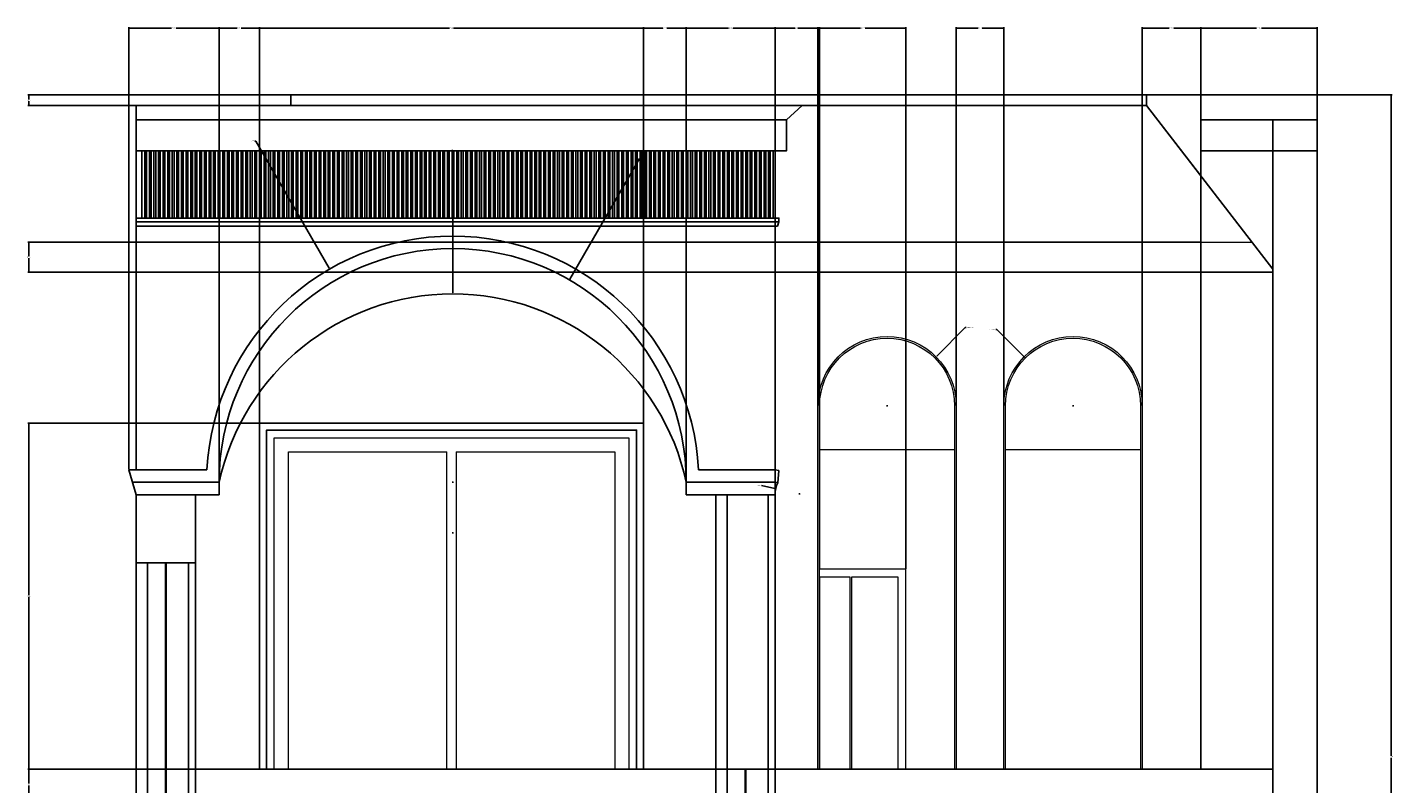
# Model space of a CAD drawing. Units: feet. Extents: x 2352 to 2983, y 950 to 1233.
# Tile 5 of 5: x 2718 to 2983, y 1086 to 1233. Entities that reach past the tile are written whole.
import ezdxf

# ---------------------------------------------------------------- set-up
doc = ezdxf.new("R2010")
doc.units = ezdxf.units.FT
for name, color, linetype, lineweight in [('A-ANNO-DIMS', 2, 'Continuous', 18), ('A-ELEV', 7, 'Continuous', 25), ('A-GLAZ', 4, 'Continuous', 18)]:
    doc.layers.add(name, color=color, linetype=linetype, lineweight=lineweight)
doc.styles.get("Standard").update_dxf_attribs({"font": 'arial.ttf'})
doc.dimstyles.get("Standard").update_dxf_attribs({"dimtxt": 0.18, "dimasz": 0.18, "dimexe": 0.18, "dimexo": 0.0625, "dimgap": 0.09, "dimtad": 0, "dimtih": 1, "dimtoh": 1, "dimdec": 1, "dimzin": 0, "dimdsep": 46, "dimlunit": 3, "dimtxsty": 'Standard', "dimcen": 0.09, "dimadec": 0, "dimazin": 0, "dimtfac": 1, "dimtdec": 1, "dimtofl": 0, "dimtmove": 0, "dimatfit": 3, "dimfxl": 1, "dimtolj": 1, "dimtzin": 0, "dimarcsym": 0})

# ---------------------------------------------------------------- blocks, each defined once
blk = doc.blocks.new('*D30')
at = {"layer": 'A-ANNO-DIMS', "color": 0, "lineweight": -2, "transparency": 16777216}
for p, q in [((2934.99, 1219.82), (2982.56, 1219.82)), ((2982.38, 1219.64), (2982.38, 1091.6)), ((2982.38, 963.19), (2982.38, 1091.23)), ((2969.32, 963.01), (2982.56, 963.01))]:
    blk.add_line(p, q, dxfattribs=at)
at = {"layer": 'A-ANNO-DIMS', "color": 0, "transparency": 16777216}
for points in [[(2982.35, 1219.64), (2982.41, 1219.64), (2982.38, 1219.82)], [(2982.35, 963.19), (2982.41, 963.19), (2982.38, 963.01)]]:
    blk.add_solid(points, dxfattribs=at)
at = {"layer": 'Defpoints', "color": 0, "transparency": 16777216}
for p in [(2934.93, 1219.82), (2982.38, 1219.82), (2969.25, 963.01)]:
    blk.add_point(p, dxfattribs=at)
at = {"layer": 'A-ANNO-DIMS', "color": 0, "transparency": 16777216, "insert": (2982.38, 1091.42), "char_height": 0.18, "attachment_point": 5}
blk.add_mtext('\\A1;256.8', dxfattribs=at)
blk = doc.blocks.new('*D43')
at = {"layer": 'A-ANNO-DIMS', "color": 0, "lineweight": -2, "transparency": 16777216}
for p, q in [((2737.35, 1147.15), (2737.35, 1232.95)), ((2737.53, 1232.77), (2745.66, 1232.77)), ((2754.71, 1232.77), (2746.57, 1232.77)), ((2754.89, 1144.73), (2754.89, 1232.95))]:
    blk.add_line(p, q, dxfattribs=at)
at = {"layer": 'A-ANNO-DIMS', "color": 0, "transparency": 16777216}
for points in [[(2737.53, 1232.8), (2737.53, 1232.74), (2737.35, 1232.77)], [(2754.71, 1232.8), (2754.71, 1232.74), (2754.89, 1232.77)]]:
    blk.add_solid(points, dxfattribs=at)
at = {"layer": 'Defpoints', "color": 0, "transparency": 16777216}
for p in [(2754.89, 1232.77), (2737.35, 1147.09), (2754.89, 1144.67)]:
    blk.add_point(p, dxfattribs=at)
at = {"layer": 'A-ANNO-DIMS', "color": 0, "transparency": 16777216, "insert": (2746.12, 1232.77), "char_height": 0.18, "attachment_point": 5}
blk.add_mtext('\\A1;17.545', dxfattribs=at)
blk = doc.blocks.new('*D44')
at = {"layer": 'A-ANNO-DIMS', "color": 0, "lineweight": -2, "transparency": 16777216}
for p, q in [((2754.89, 1144.73), (2754.89, 1232.95)), ((2755.07, 1232.77), (2758.42, 1232.77)), ((2762.55, 1232.77), (2759.2, 1232.77)), ((2762.73, 1156.23), (2762.73, 1232.95))]:
    blk.add_line(p, q, dxfattribs=at)
at = {"layer": 'A-ANNO-DIMS', "color": 0, "transparency": 16777216}
for points in [[(2755.07, 1232.8), (2755.07, 1232.74), (2754.89, 1232.77)], [(2762.55, 1232.8), (2762.55, 1232.74), (2762.73, 1232.77)]]:
    blk.add_solid(points, dxfattribs=at)
at = {"layer": 'Defpoints', "color": 0, "transparency": 16777216}
for p in [(2762.73, 1232.77), (2762.73, 1156.16), (2754.89, 1144.67)]:
    blk.add_point(p, dxfattribs=at)
at = {"layer": 'A-ANNO-DIMS', "color": 0, "transparency": 16777216, "insert": (2758.81, 1232.77), "char_height": 0.18, "attachment_point": 5}
blk.add_mtext('\\A1;7.834', dxfattribs=at)
blk = doc.blocks.new('*D45')
at = {"layer": 'A-ANNO-DIMS', "color": 0, "lineweight": -2, "transparency": 16777216}
for p, q in [((2762.73, 1156.23), (2762.73, 1232.95)), ((2762.91, 1232.77), (2799.62, 1232.77)), ((2837.11, 1232.77), (2800.4, 1232.77)), ((2837.29, 1156.23), (2837.29, 1232.95))]:
    blk.add_line(p, q, dxfattribs=at)
at = {"layer": 'A-ANNO-DIMS', "color": 0, "transparency": 16777216}
for points in [[(2762.91, 1232.8), (2762.91, 1232.74), (2762.73, 1232.77)], [(2837.11, 1232.8), (2837.11, 1232.74), (2837.29, 1232.77)]]:
    blk.add_solid(points, dxfattribs=at)
at = {"layer": 'Defpoints', "color": 0, "transparency": 16777216}
for p in [(2837.29, 1232.77), (2762.73, 1156.16), (2837.29, 1156.16)]:
    blk.add_point(p, dxfattribs=at)
at = {"layer": 'A-ANNO-DIMS', "color": 0, "transparency": 16777216, "insert": (2800.01, 1232.77), "char_height": 0.18, "attachment_point": 5}
blk.add_mtext('\\A1;74.57', dxfattribs=at)
blk = doc.blocks.new('*D46')
at = {"layer": 'A-ANNO-DIMS', "color": 0, "lineweight": -2, "transparency": 16777216}
for p, q in [((2837.29, 1156.23), (2837.29, 1232.95)), ((2837.47, 1232.77), (2841.04, 1232.77)), ((2845.39, 1232.77), (2841.82, 1232.77)), ((2845.57, 1144.73), (2845.57, 1232.95))]:
    blk.add_line(p, q, dxfattribs=at)
at = {"layer": 'A-ANNO-DIMS', "color": 0, "transparency": 16777216}
for points in [[(2837.47, 1232.8), (2837.47, 1232.74), (2837.29, 1232.77)], [(2845.39, 1232.8), (2845.39, 1232.74), (2845.57, 1232.77)]]:
    blk.add_solid(points, dxfattribs=at)
at = {"layer": 'Defpoints', "color": 0, "transparency": 16777216}
for p in [(2845.57, 1232.77), (2837.29, 1156.16), (2845.57, 1144.67)]:
    blk.add_point(p, dxfattribs=at)
at = {"layer": 'A-ANNO-DIMS', "color": 0, "transparency": 16777216, "insert": (2841.43, 1232.77), "char_height": 0.18, "attachment_point": 5}
blk.add_mtext('\\A1;8.282', dxfattribs=at)
blk = doc.blocks.new('*D47')
at = {"layer": 'A-ANNO-DIMS', "color": 0, "lineweight": -2, "transparency": 16777216}
for p, q in [((2845.57, 1144.73), (2845.57, 1232.95)), ((2845.75, 1232.77), (2853.74, 1232.77)), ((2862.65, 1232.77), (2854.65, 1232.77)), ((2862.83, 1142.3), (2862.83, 1232.95))]:
    blk.add_line(p, q, dxfattribs=at)
at = {"layer": 'A-ANNO-DIMS', "color": 0, "transparency": 16777216}
for points in [[(2845.75, 1232.8), (2845.75, 1232.74), (2845.57, 1232.77)], [(2862.65, 1232.8), (2862.65, 1232.74), (2862.83, 1232.77)]]:
    blk.add_solid(points, dxfattribs=at)
at = {"layer": 'Defpoints', "color": 0, "transparency": 16777216}
for p in [(2862.83, 1232.77), (2845.57, 1144.67), (2862.83, 1142.24)]:
    blk.add_point(p, dxfattribs=at)
at = {"layer": 'A-ANNO-DIMS', "color": 0, "transparency": 16777216, "insert": (2854.2, 1232.77), "char_height": 0.18, "attachment_point": 5}
blk.add_mtext('\\A1;17.254', dxfattribs=at)
blk = doc.blocks.new('*D48')
at = {"layer": 'A-ANNO-DIMS', "color": 0, "lineweight": -2, "transparency": 16777216}
for p, q in [((2862.83, 1191.3), (2862.83, 1232.95)), ((2863.01, 1232.77), (2866.72, 1232.77)), ((2870.95, 1232.77), (2867.23, 1232.77)), ((2871.13, 1159.59), (2871.13, 1232.95))]:
    blk.add_line(p, q, dxfattribs=at)
at = {"layer": 'A-ANNO-DIMS', "color": 0, "transparency": 16777216}
for points in [[(2863.01, 1232.8), (2863.01, 1232.74), (2862.83, 1232.77)], [(2870.95, 1232.8), (2870.95, 1232.74), (2871.13, 1232.77)]]:
    blk.add_solid(points, dxfattribs=at)
at = {"layer": 'Defpoints', "color": 0, "transparency": 16777216}
for p in [(2871.13, 1232.77), (2862.83, 1191.24), (2871.13, 1159.53)]:
    blk.add_point(p, dxfattribs=at)
at = {"layer": 'A-ANNO-DIMS', "color": 0, "transparency": 16777216, "insert": (2866.98, 1232.77), "char_height": 0.18, "attachment_point": 5}
blk.add_mtext('\\A1;8.3', dxfattribs=at)
blk = doc.blocks.new('*D49')
at = {"layer": 'A-ANNO-DIMS', "color": 0, "lineweight": -2, "transparency": 16777216}
for p, q in [((2871.45, 1127.84), (2871.45, 1232.95)), ((2871.63, 1232.77), (2879.36, 1232.77)), ((2887.99, 1232.77), (2880.27, 1232.77)), ((2888.17, 1127.84), (2888.17, 1232.95))]:
    blk.add_line(p, q, dxfattribs=at)
at = {"layer": 'A-ANNO-DIMS', "color": 0, "transparency": 16777216}
for points in [[(2871.63, 1232.8), (2871.63, 1232.74), (2871.45, 1232.77)], [(2887.99, 1232.8), (2887.99, 1232.74), (2888.17, 1232.77)]]:
    blk.add_solid(points, dxfattribs=at)
at = {"layer": 'Defpoints', "color": 0, "transparency": 16777216}
for p in [(2888.17, 1232.77), (2871.45, 1127.78), (2888.17, 1127.78)]:
    blk.add_point(p, dxfattribs=at)
at = {"layer": 'A-ANNO-DIMS', "color": 0, "transparency": 16777216, "insert": (2879.81, 1232.77), "char_height": 0.18, "attachment_point": 5}
blk.add_mtext('\\A1;16.717', dxfattribs=at)
blk = doc.blocks.new('*D50')
at = {"layer": 'A-ANNO-DIMS', "color": 0, "lineweight": -2, "transparency": 16777216}
for p, q in [((2897.97, 1159.59), (2897.97, 1232.95)), ((2898.15, 1232.77), (2902.2, 1232.77)), ((2907.04, 1232.77), (2902.99, 1232.77)), ((2907.22, 1159.59), (2907.22, 1232.95))]:
    blk.add_line(p, q, dxfattribs=at)
at = {"layer": 'A-ANNO-DIMS', "color": 0, "transparency": 16777216}
for points in [[(2898.15, 1232.8), (2898.15, 1232.74), (2897.97, 1232.77)], [(2907.04, 1232.8), (2907.04, 1232.74), (2907.22, 1232.77)]]:
    blk.add_solid(points, dxfattribs=at)
at = {"layer": 'Defpoints', "color": 0, "transparency": 16777216}
for p in [(2907.22, 1232.77), (2897.97, 1159.53), (2907.22, 1159.53)]:
    blk.add_point(p, dxfattribs=at)
at = {"layer": 'A-ANNO-DIMS', "color": 0, "transparency": 16777216, "insert": (2902.59, 1232.77), "char_height": 0.18, "attachment_point": 5}
blk.add_mtext('\\A1;9.249', dxfattribs=at)
blk = doc.blocks.new('*D51')
at = {"layer": 'A-ANNO-DIMS', "color": 0, "lineweight": -2, "transparency": 16777216}
for p, q in [((2934.06, 1159.59), (2934.06, 1232.95)), ((2934.24, 1232.77), (2939.3, 1232.77)), ((2945.28, 1232.77), (2940.22, 1232.77)), ((2945.46, 1185.51), (2945.46, 1232.95))]:
    blk.add_line(p, q, dxfattribs=at)
at = {"layer": 'A-ANNO-DIMS', "color": 0, "transparency": 16777216}
for points in [[(2934.24, 1232.8), (2934.24, 1232.74), (2934.06, 1232.77)], [(2945.28, 1232.8), (2945.28, 1232.74), (2945.46, 1232.77)]]:
    blk.add_solid(points, dxfattribs=at)
at = {"layer": 'Defpoints', "color": 0, "transparency": 16777216}
for p in [(2945.46, 1232.77), (2945.46, 1185.45), (2934.06, 1159.53)]:
    blk.add_point(p, dxfattribs=at)
at = {"layer": 'A-ANNO-DIMS', "color": 0, "transparency": 16777216, "insert": (2939.76, 1232.77), "char_height": 0.18, "attachment_point": 5}
blk.add_mtext('\\A1;11.395', dxfattribs=at)
blk = doc.blocks.new('*D52')
at = {"layer": 'A-ANNO-DIMS', "color": 0, "lineweight": -2, "transparency": 16777216}
for p, q in [((2945.46, 1215.08), (2945.46, 1232.95)), ((2945.64, 1232.77), (2956.27, 1232.77)), ((2967.83, 1232.77), (2957.2, 1232.77)), ((2968.01, 1215.08), (2968.01, 1232.95))]:
    blk.add_line(p, q, dxfattribs=at)
at = {"layer": 'A-ANNO-DIMS', "color": 0, "transparency": 16777216}
for points in [[(2945.64, 1232.8), (2945.64, 1232.74), (2945.46, 1232.77)], [(2967.83, 1232.8), (2967.83, 1232.74), (2968.01, 1232.77)]]:
    blk.add_solid(points, dxfattribs=at)
at = {"layer": 'Defpoints', "color": 0, "transparency": 16777216}
for p in [(2968.01, 1232.77), (2945.46, 1215.01), (2968.01, 1215.01)]:
    blk.add_point(p, dxfattribs=at)
at = {"layer": 'A-ANNO-DIMS', "color": 0, "transparency": 16777216, "insert": (2956.74, 1232.77), "char_height": 0.18, "attachment_point": 5}
blk.add_mtext('\\A1;22.554', dxfattribs=at)
blk = doc.blocks.new('*D56')
at = {"layer": 'A-ANNO-DIMS', "color": 0, "lineweight": -2, "transparency": 16777216}
for p, q in [((2750.25, 1089.01), (2717.79, 1089.01)), ((2717.97, 1088.83), (2717.97, 1086.19)), ((2717.97, 1083.19), (2717.97, 1085.83)), ((2748.9, 1083.01), (2717.79, 1083.01))]:
    blk.add_line(p, q, dxfattribs=at)
at = {"layer": 'A-ANNO-DIMS', "color": 0, "transparency": 16777216}
for points in [[(2717.94, 1088.83), (2718, 1088.83), (2717.97, 1089.01)], [(2717.94, 1083.19), (2718, 1083.19), (2717.97, 1083.01)]]:
    blk.add_solid(points, dxfattribs=at)
at = {"layer": 'Defpoints', "color": 0, "transparency": 16777216}
for p in [(2717.97, 1089.01), (2750.31, 1089.01), (2748.96, 1083.01)]:
    blk.add_point(p, dxfattribs=at)
at = {"layer": 'A-ANNO-DIMS', "color": 0, "transparency": 16777216, "insert": (2717.97, 1086.01), "char_height": 0.18, "attachment_point": 5}
blk.add_mtext('\\A1;6', dxfattribs=at)
blk = doc.blocks.new('*D57')
at = {"layer": 'A-ANNO-DIMS', "color": 0, "lineweight": -2, "transparency": 16777216}
for p, q in [((2762.66, 1156.16), (2717.79, 1156.16)), ((2717.97, 1155.98), (2717.97, 1122.77)), ((2717.97, 1089.19), (2717.97, 1122.41)), ((2762.66, 1089.01), (2717.79, 1089.01))]:
    blk.add_line(p, q, dxfattribs=at)
at = {"layer": 'A-ANNO-DIMS', "color": 0, "transparency": 16777216}
for points in [[(2717.94, 1155.98), (2718, 1155.98), (2717.97, 1156.16)], [(2717.94, 1089.19), (2718, 1089.19), (2717.97, 1089.01)]]:
    blk.add_solid(points, dxfattribs=at)
at = {"layer": 'Defpoints', "color": 0, "transparency": 16777216}
for p in [(2717.97, 1156.16), (2762.73, 1156.16), (2762.73, 1089.01)]:
    blk.add_point(p, dxfattribs=at)
at = {"layer": 'A-ANNO-DIMS', "color": 0, "transparency": 16777216, "insert": (2717.97, 1122.59), "char_height": 0.18, "attachment_point": 5}
blk.add_mtext('\\A1;67.15', dxfattribs=at)
blk = doc.blocks.new('*D58')
at = {"layer": 'A-ANNO-DIMS', "color": 0, "lineweight": -2, "transparency": 16777216}
for p, q in [((2862.76, 1191.24), (2717.79, 1191.24)), ((2717.97, 1191.06), (2717.97, 1188.52)), ((2717.97, 1185.63), (2717.97, 1188.16)), ((2862.76, 1185.45), (2717.79, 1185.45))]:
    blk.add_line(p, q, dxfattribs=at)
at = {"layer": 'A-ANNO-DIMS', "color": 0, "transparency": 16777216}
for points in [[(2717.94, 1191.06), (2718, 1191.06), (2717.97, 1191.24)], [(2717.94, 1185.63), (2718, 1185.63), (2717.97, 1185.45)]]:
    blk.add_solid(points, dxfattribs=at)
at = {"layer": 'Defpoints', "color": 0, "transparency": 16777216}
for p in [(2717.97, 1191.24), (2862.83, 1191.24), (2862.83, 1185.45)]:
    blk.add_point(p, dxfattribs=at)
at = {"layer": 'A-ANNO-DIMS', "color": 0, "transparency": 16777216, "insert": (2717.97, 1188.34), "char_height": 0.18, "attachment_point": 5}
blk.add_mtext('\\A1;5.788', dxfattribs=at)
blk = doc.blocks.new('*D59')
at = {"layer": 'A-ANNO-DIMS', "color": 0, "lineweight": -2, "transparency": 16777216}
for p, q in [((2768.76, 1219.82), (2717.79, 1219.82)), ((2717.97, 1219.64), (2717.97, 1218.97)), ((2768.76, 1217.75), (2717.79, 1217.75)), ((2717.97, 1217.93), (2717.97, 1218.6))]:
    blk.add_line(p, q, dxfattribs=at)
at = {"layer": 'A-ANNO-DIMS', "color": 0, "transparency": 16777216}
for points in [[(2717.94, 1219.64), (2718, 1219.64), (2717.97, 1219.82)], [(2717.94, 1217.93), (2718, 1217.93), (2717.97, 1217.75)]]:
    blk.add_solid(points, dxfattribs=at)
at = {"layer": 'Defpoints', "color": 0, "transparency": 16777216}
for p in [(2717.97, 1219.82), (2768.82, 1219.82), (2768.82, 1217.75)]:
    blk.add_point(p, dxfattribs=at)
at = {"layer": 'A-ANNO-DIMS', "color": 0, "transparency": 16777216, "insert": (2717.97, 1218.78), "char_height": 0.18, "attachment_point": 5}
blk.add_mtext('\\A1;2.067', dxfattribs=at)
blk = doc.blocks.new('*D67')
at = {"layer": 'A-ANNO-DIMS', "color": 0, "lineweight": -2, "transparency": 16777216}
for p, q in [((2761.84, 1210.85), (2762.02, 1210.85)), ((2762.02, 1210.85), (2776.26, 1186.19)), ((2800.14, 1144.67), (2800.32, 1144.67)), ((2800.23, 1144.58), (2800.23, 1144.76))]:
    blk.add_line(p, q, dxfattribs=at)
at = {"layer": 'A-ANNO-DIMS', "color": 0, "transparency": 16777216}
blk.add_solid([(2776.28, 1186.2), (2776.23, 1186.17), (2776.35, 1186.03)], dxfattribs=at)
at = {"layer": 'Defpoints', "color": 0, "transparency": 16777216}
for p in [(2776.35, 1186.03), (2800.23, 1144.67)]:
    blk.add_point(p, dxfattribs=at)
at = {"layer": 'A-ANNO-DIMS', "color": 0, "transparency": 16777216, "insert": (2761.36, 1210.85), "char_height": 0.18, "attachment_point": 5}
blk.add_mtext('\\A1;R47.77', dxfattribs=at)
blk = doc.blocks.new('*D68')
at = {"layer": 'A-ANNO-DIMS', "color": 0, "lineweight": -2, "transparency": 16777216}
for p, q in [((2800.05, 1209.06), (2800.23, 1209.06)), ((2800.23, 1209.06), (2800.23, 1181.4)), ((2800.14, 1134.83), (2800.32, 1134.83)), ((2800.23, 1134.74), (2800.23, 1134.92))]:
    blk.add_line(p, q, dxfattribs=at)
at = {"layer": 'A-ANNO-DIMS', "color": 0, "transparency": 16777216}
blk.add_solid([(2800.26, 1181.4), (2800.2, 1181.4), (2800.23, 1181.22)], dxfattribs=at)
at = {"layer": 'Defpoints', "color": 0, "transparency": 16777216}
for p in [(2800.23, 1181.22), (2800.23, 1134.83)]:
    blk.add_point(p, dxfattribs=at)
at = {"layer": 'A-ANNO-DIMS', "color": 0, "transparency": 16777216, "insert": (2799.64, 1209.06), "char_height": 0.18, "attachment_point": 5}
blk.add_mtext('\\A1;R46.4', dxfattribs=at)
blk = doc.blocks.new('*D69')
at = {"layer": 'A-ANNO-DIMS', "color": 0, "lineweight": -2, "transparency": 16777216}
for p, q in [((2836.5, 1207.49), (2822.99, 1184.09)), ((2836.68, 1207.49), (2836.5, 1207.49)), ((2800.14, 1144.67), (2800.32, 1144.67)), ((2800.23, 1144.58), (2800.23, 1144.76))]:
    blk.add_line(p, q, dxfattribs=at)
at = {"layer": 'A-ANNO-DIMS', "color": 0, "transparency": 16777216}
blk.add_solid([(2822.97, 1184.1), (2823.02, 1184.07), (2822.9, 1183.93)], dxfattribs=at)
at = {"layer": 'Defpoints', "color": 0, "transparency": 16777216}
for p in [(2822.9, 1183.93), (2800.23, 1144.67)]:
    blk.add_point(p, dxfattribs=at)
at = {"layer": 'A-ANNO-DIMS', "color": 0, "transparency": 16777216, "insert": (2837.16, 1207.49), "char_height": 0.18, "attachment_point": 5}
blk.add_mtext('\\A1;R45.34', dxfattribs=at)
blk = doc.blocks.new('*D72')
at = {"layer": 'A-ANNO-DIMS', "color": 0, "lineweight": -2, "transparency": 16777216}
for p, q in [((2899.73, 1174.71), (2894.17, 1169.15)), ((2899.91, 1174.71), (2899.73, 1174.71)), ((2884.46, 1159.53), (2884.64, 1159.53)), ((2884.55, 1159.44), (2884.55, 1159.62))]:
    blk.add_line(p, q, dxfattribs=at)
at = {"layer": 'A-ANNO-DIMS', "color": 0, "transparency": 16777216}
blk.add_solid([(2894.14, 1169.17), (2894.19, 1169.12), (2894.04, 1169.02)], dxfattribs=at)
at = {"layer": 'Defpoints', "color": 0, "transparency": 16777216}
for p in [(2894.04, 1169.02), (2884.55, 1159.53)]:
    blk.add_point(p, dxfattribs=at)
at = {"layer": 'A-ANNO-DIMS', "color": 0, "transparency": 16777216, "insert": (2900.66, 1174.71), "char_height": 0.18, "attachment_point": 5}
blk.add_mtext('\\A1;2X R13.422', dxfattribs=at)
blk = doc.blocks.new('*D73')
at = {"layer": 'A-ANNO-DIMS', "color": 0, "lineweight": -2, "transparency": 16777216}
for p, q in [((2905.65, 1174.34), (2905.83, 1174.34)), ((2905.83, 1174.34), (2911.26, 1168.91)), ((2920.55, 1159.53), (2920.73, 1159.53)), ((2920.64, 1159.44), (2920.64, 1159.62))]:
    blk.add_line(p, q, dxfattribs=at)
at = {"layer": 'A-ANNO-DIMS', "color": 0, "transparency": 16777216}
blk.add_solid([(2911.28, 1168.94), (2911.23, 1168.89), (2911.38, 1168.79)], dxfattribs=at)
at = {"layer": 'Defpoints', "color": 0, "transparency": 16777216}
for p in [(2911.38, 1168.79), (2920.64, 1159.53)]:
    blk.add_point(p, dxfattribs=at)
at = {"layer": 'A-ANNO-DIMS', "color": 0, "transparency": 16777216, "insert": (2904.9, 1174.34), "char_height": 0.18, "attachment_point": 5}
blk.add_mtext('\\A1;2X R13.094', dxfattribs=at)
blk = doc.blocks.new('*D74')
at = {"layer": 'A-ANNO-DIMS', "color": 0, "lineweight": -2, "transparency": 16777216}
for p, q in [((2860.19, 1144.07), (2862.76, 1143.48)), ((2867.43, 1142.41), (2867.61, 1142.41)), ((2867.52, 1142.32), (2867.52, 1142.5))]:
    blk.add_line(p, q, dxfattribs=at)
at = {"layer": 'A-ANNO-DIMS', "color": 0, "transparency": 16777216}
blk.add_solid([(2862.77, 1143.51), (2862.76, 1143.45), (2862.94, 1143.44)], dxfattribs=at)
at = {"layer": 'Defpoints', "color": 0, "transparency": 16777216}
for p in [(2862.94, 1143.44), (2867.52, 1142.41)]:
    blk.add_point(p, dxfattribs=at)
at = {"layer": 'A-ANNO-DIMS', "color": 0, "transparency": 16777216, "insert": (2859.71, 1144.07), "char_height": 0.18, "attachment_point": 5}
blk.add_mtext('\\A1;R4.699', dxfattribs=at)

msp = doc.modelspace()

# ---------------------------------------------------------------- linework, layer by layer
at = {"layer": 'A-ELEV'}
for p, q in [((2865.0307, 1215.0126), (2868.0927, 1217.7513)), ((2934.9257, 1217.7513), (2945.4584, 1204.1231)), ((2934.9257, 1217.7513), (2959.4504, 1186.0189)), ((2865.0307, 1215.0126), (2738.7806, 1215.0126)), ((2968.0127, 1215.0126), (2945.4584, 1215.0126)), ((2945.4584, 1204.1231), (2945.4584, 1215.0126)), ((2738.7806, 1209.0126), (2865.0307, 1209.0126)), ((2862.8263, 1195.936), (2862.8263, 1209.0126)), ((2945.4584, 1209.0126), (2968.0127, 1209.0126)), ((2862.8263, 1194.3715), (2738.7806, 1194.3715)), ((2862.8263, 1147.0918), (2862.8263, 1194.3715)), ((2863.2863, 1194.3715), (2862.8263, 1194.3715)), ((2863.5613, 1195.1775), (2863.2863, 1194.3715)), ((2862.8263, 1191.2362), (2945.4584, 1191.2362)), ((2945.4584, 1191.2362), (2955.4573, 1191.1856)), ((2862.8263, 1185.4477), (2945.4584, 1185.4477)), ((2945.4584, 1089.0126), (2945.4584, 1185.4477)), ((2945.4584, 1185.4477), (2959.4504, 1185.4477)), ((2738.7806, 1147.0918), (2737.3463, 1147.0918)), ((2737.3463, 1147.0918), (2738.7806, 1142.2389)), ((2752.527, 1147.0918), (2738.7806, 1147.0918)), ((2847.9373, 1147.0918), (2862.8263, 1147.0918)), ((2862.8263, 1147.0918), (2863.5417, 1146.9764)), ((2863.5417, 1146.9764), (2863.3566, 1144.5798)), ((2754.8917, 1144.6653), (2738.0635, 1144.6653)), ((2754.8917, 1144.6653), (2754.8917, 1142.2389)), ((2845.5725, 1144.6653), (2862.8263, 1144.6653)), ((2845.5725, 1144.6653), (2845.5725, 1142.2389)), ((2862.8263, 1144.6653), (2863.3566, 1144.5798)), ((2754.8917, 1142.2389), (2738.7806, 1142.2389)), ((2845.5725, 1142.2389), (2862.8263, 1142.2389)), ((2738.7806, 1129.0147), (2750.3114, 1129.0147)), ((2851.2955, 1089.0126), (2750.3114, 1089.0126)), ((2851.2955, 1089.0126), (2862.8263, 1089.0126)), ((2959.4504, 1089.0126), (2862.8263, 1089.0126))]:
    msp.add_line(p, q, dxfattribs=at)
for points in [[(2768.821, 1217.7513), (2934.9257, 1217.7513), (2934.9257, 1219.8182), (2768.821, 1219.8182)], [(2738.7806, 1215.0126), (2865.0307, 1215.0126), (2865.0307, 1209.0126), (2738.7806, 1209.0126)], [(2738.7806, 1209.0126), (2862.8263, 1209.0126), (2862.8263, 1195.936), (2738.7806, 1195.936)], [(2739.9081, 1209.0126), (2740.4657, 1209.0126), (2740.4657, 1195.936), (2739.9081, 1195.936)], [(2740.7984, 1209.0126), (2741.356, 1209.0126), (2741.356, 1195.936), (2740.7984, 1195.936)], [(2741.6887, 1209.0126), (2742.2464, 1209.0126), (2742.2464, 1195.936), (2741.6887, 1195.936)], [(2742.5791, 1209.0126), (2743.1367, 1209.0126), (2743.1367, 1195.936), (2742.5791, 1195.936)], [(2743.4694, 1209.0126), (2744.027, 1209.0126), (2744.027, 1195.936), (2743.4694, 1195.936)], [(2744.3597, 1209.0126), (2744.9173, 1209.0126), (2744.9173, 1195.936), (2744.3597, 1195.936)], [(2745.2501, 1209.0126), (2745.8077, 1209.0126), (2745.8077, 1195.936), (2745.2501, 1195.936)], [(2746.1404, 1209.0126), (2746.698, 1209.0126), (2746.698, 1195.936), (2746.1404, 1195.936)], [(2747.0307, 1209.0126), (2747.5883, 1209.0126), (2747.5883, 1195.936), (2747.0307, 1195.936)], [(2747.9211, 1209.0126), (2748.4787, 1209.0126), (2748.4787, 1195.936), (2747.9211, 1195.936)], [(2748.8114, 1209.0126), (2749.369, 1209.0126), (2749.369, 1195.936), (2748.8114, 1195.936)], [(2749.7017, 1209.0126), (2750.2593, 1209.0126), (2750.2593, 1195.936), (2749.7017, 1195.936)], [(2750.5921, 1209.0126), (2751.1497, 1209.0126), (2751.1497, 1195.936), (2750.5921, 1195.936)], [(2751.4824, 1209.0126), (2752.04, 1209.0126), (2752.04, 1195.936), (2751.4824, 1195.936)], [(2752.3727, 1209.0126), (2752.9303, 1209.0126), (2752.9303, 1195.936), (2752.3727, 1195.936)], [(2753.263, 1209.0126), (2753.8207, 1209.0126), (2753.8207, 1195.936), (2753.263, 1195.936)], [(2754.1534, 1209.0126), (2754.711, 1209.0126), (2754.711, 1195.936), (2754.1534, 1195.936)], [(2755.0437, 1209.0126), (2755.6013, 1209.0126), (2755.6013, 1195.936), (2755.0437, 1195.936)], [(2755.934, 1209.0126), (2756.4917, 1209.0126), (2756.4917, 1195.936), (2755.934, 1195.936)], [(2756.8244, 1209.0126), (2757.382, 1209.0126), (2757.382, 1195.936), (2756.8244, 1195.936)], [(2757.7147, 1209.0126), (2758.2723, 1209.0126), (2758.2723, 1195.936), (2757.7147, 1195.936)], [(2758.605, 1209.0126), (2759.1627, 1209.0126), (2759.1627, 1195.936), (2758.605, 1195.936)], [(2759.4954, 1209.0126), (2760.053, 1209.0126), (2760.053, 1195.936), (2759.4954, 1195.936)], [(2760.3857, 1209.0126), (2760.9433, 1209.0126), (2760.9433, 1195.936), (2760.3857, 1195.936)], [(2761.276, 1209.0126), (2761.8337, 1209.0126), (2761.8337, 1195.936), (2761.276, 1195.936)], [(2762.1664, 1209.0126), (2762.724, 1209.0126), (2762.724, 1195.936), (2762.1664, 1195.936)], [(2763.0567, 1209.0126), (2763.6143, 1209.0126), (2763.6143, 1195.936), (2763.0567, 1195.936)], [(2763.947, 1209.0126), (2764.5047, 1209.0126), (2764.5047, 1195.936), (2763.947, 1195.936)], [(2764.8374, 1209.0126), (2765.395, 1209.0126), (2765.395, 1195.936), (2764.8374, 1195.936)], [(2765.7277, 1209.0126), (2766.2853, 1209.0126), (2766.2853, 1195.936), (2765.7277, 1195.936)], [(2766.618, 1209.0126), (2767.1757, 1209.0126), (2767.1757, 1195.936), (2766.618, 1195.936)], [(2767.5084, 1209.0126), (2768.066, 1209.0126), (2768.066, 1195.936), (2767.5084, 1195.936)], [(2768.3987, 1209.0126), (2768.9563, 1209.0126), (2768.9563, 1195.936), (2768.3987, 1195.936)], [(2769.289, 1209.0126), (2769.8467, 1209.0126), (2769.8467, 1195.936), (2769.289, 1195.936)], [(2770.1794, 1209.0126), (2770.737, 1209.0126), (2770.737, 1195.936), (2770.1794, 1195.936)], [(2771.0697, 1209.0126), (2771.6273, 1209.0126), (2771.6273, 1195.936), (2771.0697, 1195.936)], [(2771.96, 1209.0126), (2772.5177, 1209.0126), (2772.5177, 1195.936), (2771.96, 1195.936)], [(2772.8504, 1209.0126), (2773.408, 1209.0126), (2773.408, 1195.936), (2772.8504, 1195.936)], [(2773.7407, 1209.0126), (2774.2983, 1209.0126), (2774.2983, 1195.936), (2773.7407, 1195.936)], [(2774.631, 1209.0126), (2775.1887, 1209.0126), (2775.1887, 1195.936), (2774.631, 1195.936)], [(2775.5214, 1209.0126), (2776.079, 1209.0126), (2776.079, 1195.936), (2775.5214, 1195.936)], [(2776.4117, 1209.0126), (2776.9693, 1209.0126), (2776.9693, 1195.936), (2776.4117, 1195.936)], [(2777.302, 1209.0126), (2777.8597, 1209.0126), (2777.8597, 1195.936), (2777.302, 1195.936)], [(2778.1924, 1209.0126), (2778.75, 1209.0126), (2778.75, 1195.936), (2778.1924, 1195.936)], [(2779.0827, 1209.0126), (2779.6403, 1209.0126), (2779.6403, 1195.936), (2779.0827, 1195.936)], [(2779.973, 1209.0126), (2780.5307, 1209.0126), (2780.5307, 1195.936), (2779.973, 1195.936)], [(2780.8634, 1209.0126), (2781.421, 1209.0126), (2781.421, 1195.936), (2780.8634, 1195.936)], [(2781.7537, 1209.0126), (2782.3113, 1209.0126), (2782.3113, 1195.936), (2781.7537, 1195.936)], [(2782.644, 1209.0126), (2783.2017, 1209.0126), (2783.2017, 1195.936), (2782.644, 1195.936)], [(2783.5344, 1209.0126), (2784.092, 1209.0126), (2784.092, 1195.936), (2783.5344, 1195.936)], [(2784.4247, 1209.0126), (2784.9823, 1209.0126), (2784.9823, 1195.936), (2784.4247, 1195.936)], [(2785.315, 1209.0126), (2785.8727, 1209.0126), (2785.8727, 1195.936), (2785.315, 1195.936)], [(2786.2054, 1209.0126), (2786.763, 1209.0126), (2786.763, 1195.936), (2786.2054, 1195.936)], [(2787.0957, 1209.0126), (2787.6533, 1209.0126), (2787.6533, 1195.936), (2787.0957, 1195.936)], [(2787.986, 1209.0126), (2788.5437, 1209.0126), (2788.5437, 1195.936), (2787.986, 1195.936)], [(2788.8764, 1209.0126), (2789.434, 1209.0126), (2789.434, 1195.936), (2788.8764, 1195.936)], [(2789.7667, 1209.0126), (2790.3243, 1209.0126), (2790.3243, 1195.936), (2789.7667, 1195.936)], [(2790.657, 1209.0126), (2791.2147, 1209.0126), (2791.2147, 1195.936), (2790.657, 1195.936)], [(2791.5474, 1209.0126), (2792.105, 1209.0126), (2792.105, 1195.936), (2791.5474, 1195.936)], [(2792.4377, 1209.0126), (2792.9953, 1209.0126), (2792.9953, 1195.936), (2792.4377, 1195.936)], [(2793.328, 1209.0126), (2793.8856, 1209.0126), (2793.8856, 1195.936), (2793.328, 1195.936)], [(2794.2184, 1209.0126), (2794.776, 1209.0126), (2794.776, 1195.936), (2794.2184, 1195.936)], [(2795.1087, 1209.0126), (2795.6663, 1209.0126), (2795.6663, 1195.936), (2795.1087, 1195.936)], [(2795.999, 1209.0126), (2796.5566, 1209.0126), (2796.5566, 1195.936), (2795.999, 1195.936)], [(2796.8894, 1209.0126), (2797.447, 1209.0126), (2797.447, 1195.936), (2796.8894, 1195.936)], [(2797.7797, 1209.0126), (2798.3373, 1209.0126), (2798.3373, 1195.936), (2797.7797, 1195.936)], [(2798.67, 1209.0126), (2799.2276, 1209.0126), (2799.2276, 1195.936), (2798.67, 1195.936)], [(2799.5604, 1209.0126), (2800.118, 1209.0126), (2800.118, 1195.936), (2799.5604, 1195.936)], [(2800.4507, 1209.0126), (2801.0083, 1209.0126), (2801.0083, 1195.936), (2800.4507, 1195.936)], [(2801.341, 1209.0126), (2801.8986, 1209.0126), (2801.8986, 1195.936), (2801.341, 1195.936)], [(2802.2313, 1209.0126), (2802.789, 1209.0126), (2802.789, 1195.936), (2802.2313, 1195.936)], [(2803.1217, 1209.0126), (2803.6793, 1209.0126), (2803.6793, 1195.936), (2803.1217, 1195.936)], [(2804.012, 1209.0126), (2804.5696, 1209.0126), (2804.5696, 1195.936), (2804.012, 1195.936)], [(2804.9023, 1209.0126), (2805.46, 1209.0126), (2805.46, 1195.936), (2804.9023, 1195.936)], [(2805.7927, 1209.0126), (2806.3503, 1209.0126), (2806.3503, 1195.936), (2805.7927, 1195.936)], [(2806.683, 1209.0126), (2807.2406, 1209.0126), (2807.2406, 1195.936), (2806.683, 1195.936)], [(2807.5733, 1209.0126), (2808.131, 1209.0126), (2808.131, 1195.936), (2807.5733, 1195.936)], [(2808.4637, 1209.0126), (2809.0213, 1209.0126), (2809.0213, 1195.936), (2808.4637, 1195.936)], [(2809.354, 1209.0126), (2809.9116, 1209.0126), (2809.9116, 1195.936), (2809.354, 1195.936)], [(2810.2443, 1209.0126), (2810.802, 1209.0126), (2810.802, 1195.936), (2810.2443, 1195.936)], [(2811.1347, 1209.0126), (2811.6923, 1209.0126), (2811.6923, 1195.936), (2811.1347, 1195.936)], [(2812.025, 1209.0126), (2812.5826, 1209.0126), (2812.5826, 1195.936), (2812.025, 1195.936)], [(2812.9153, 1209.0126), (2813.473, 1209.0126), (2813.473, 1195.936), (2812.9153, 1195.936)], [(2813.8057, 1209.0126), (2814.3633, 1209.0126), (2814.3633, 1195.936), (2813.8057, 1195.936)], [(2814.696, 1209.0126), (2815.2536, 1209.0126), (2815.2536, 1195.936), (2814.696, 1195.936)], [(2815.5863, 1209.0126), (2816.144, 1209.0126), (2816.144, 1195.936), (2815.5863, 1195.936)], [(2816.4767, 1209.0126), (2817.0343, 1209.0126), (2817.0343, 1195.936), (2816.4767, 1195.936)], [(2817.367, 1209.0126), (2817.9246, 1209.0126), (2817.9246, 1195.936), (2817.367, 1195.936)], [(2818.2573, 1209.0126), (2818.815, 1209.0126), (2818.815, 1195.936), (2818.2573, 1195.936)], [(2819.1477, 1209.0126), (2819.7053, 1209.0126), (2819.7053, 1195.936), (2819.1477, 1195.936)], [(2820.038, 1209.0126), (2820.5956, 1209.0126), (2820.5956, 1195.936), (2820.038, 1195.936)], [(2820.9283, 1209.0126), (2821.486, 1209.0126), (2821.486, 1195.936), (2820.9283, 1195.936)], [(2821.8187, 1209.0126), (2822.3763, 1209.0126), (2822.3763, 1195.936), (2821.8187, 1195.936)], [(2822.709, 1209.0126), (2823.2666, 1209.0126), (2823.2666, 1195.936), (2822.709, 1195.936)], [(2823.5993, 1209.0126), (2824.157, 1209.0126), (2824.157, 1195.936), (2823.5993, 1195.936)], [(2824.4897, 1209.0126), (2825.0473, 1209.0126), (2825.0473, 1195.936), (2824.4897, 1195.936)], [(2825.38, 1209.0126), (2825.9376, 1209.0126), (2825.9376, 1195.936), (2825.38, 1195.936)], [(2826.2703, 1209.0126), (2826.828, 1209.0126), (2826.828, 1195.936), (2826.2703, 1195.936)], [(2827.1607, 1209.0126), (2827.7183, 1209.0126), (2827.7183, 1195.936), (2827.1607, 1195.936)], [(2828.051, 1209.0126), (2828.6086, 1209.0126), (2828.6086, 1195.936), (2828.051, 1195.936)], [(2828.9413, 1209.0126), (2829.499, 1209.0126), (2829.499, 1195.936), (2828.9413, 1195.936)], [(2829.8317, 1209.0126), (2830.3893, 1209.0126), (2830.3893, 1195.936), (2829.8317, 1195.936)], [(2830.722, 1209.0126), (2831.2796, 1209.0126), (2831.2796, 1195.936), (2830.722, 1195.936)], [(2831.6123, 1209.0126), (2832.17, 1209.0126), (2832.17, 1195.936), (2831.6123, 1195.936)], [(2832.5027, 1209.0126), (2833.0603, 1209.0126), (2833.0603, 1195.936), (2832.5027, 1195.936)], [(2833.393, 1209.0126), (2833.9506, 1209.0126), (2833.9506, 1195.936), (2833.393, 1195.936)], [(2834.2833, 1209.0126), (2834.841, 1209.0126), (2834.841, 1195.936), (2834.2833, 1195.936)], [(2835.1737, 1209.0126), (2835.7313, 1209.0126), (2835.7313, 1195.936), (2835.1737, 1195.936)], [(2836.064, 1209.0126), (2836.6216, 1209.0126), (2836.6216, 1195.936), (2836.064, 1195.936)], [(2836.9543, 1209.0126), (2837.512, 1209.0126), (2837.512, 1195.936), (2836.9543, 1195.936)], [(2837.8447, 1209.0126), (2838.4023, 1209.0126), (2838.4023, 1195.936), (2837.8447, 1195.936)], [(2838.735, 1209.0126), (2839.2926, 1209.0126), (2839.2926, 1195.936), (2838.735, 1195.936)], [(2839.6253, 1209.0126), (2840.183, 1209.0126), (2840.183, 1195.936), (2839.6253, 1195.936)], [(2840.5157, 1209.0126), (2841.0733, 1209.0126), (2841.0733, 1195.936), (2840.5157, 1195.936)], [(2841.406, 1209.0126), (2841.9636, 1209.0126), (2841.9636, 1195.936), (2841.406, 1195.936)], [(2842.2963, 1209.0126), (2842.8539, 1209.0126), (2842.8539, 1195.936), (2842.2963, 1195.936)], [(2843.1867, 1209.0126), (2843.7443, 1209.0126), (2843.7443, 1195.936), (2843.1867, 1195.936)], [(2844.077, 1209.0126), (2844.6346, 1209.0126), (2844.6346, 1195.936), (2844.077, 1195.936)], [(2844.9673, 1209.0126), (2845.5249, 1209.0126), (2845.5249, 1195.936), (2844.9673, 1195.936)], [(2845.8577, 1209.0126), (2846.4153, 1209.0126), (2846.4153, 1195.936), (2845.8577, 1195.936)], [(2846.748, 1209.0126), (2847.3056, 1209.0126), (2847.3056, 1195.936), (2846.748, 1195.936)], [(2847.6383, 1209.0126), (2848.1959, 1209.0126), (2848.1959, 1195.936), (2847.6383, 1195.936)], [(2848.5287, 1209.0126), (2849.0863, 1209.0126), (2849.0863, 1195.936), (2848.5287, 1195.936)], [(2849.419, 1209.0126), (2849.9766, 1209.0126), (2849.9766, 1195.936), (2849.419, 1195.936)], [(2850.3093, 1209.0126), (2850.8669, 1209.0126), (2850.8669, 1195.936), (2850.3093, 1195.936)], [(2851.1996, 1209.0126), (2851.7573, 1209.0126), (2851.7573, 1195.936), (2851.1996, 1195.936)], [(2852.09, 1209.0126), (2852.6476, 1209.0126), (2852.6476, 1195.936), (2852.09, 1195.936)], [(2852.9803, 1209.0126), (2853.5379, 1209.0126), (2853.5379, 1195.936), (2852.9803, 1195.936)], [(2853.8706, 1209.0126), (2854.4283, 1209.0126), (2854.4283, 1195.936), (2853.8706, 1195.936)], [(2854.761, 1209.0126), (2855.3186, 1209.0126), (2855.3186, 1195.936), (2854.761, 1195.936)], [(2855.6513, 1209.0126), (2856.2089, 1209.0126), (2856.2089, 1195.936), (2855.6513, 1195.936)], [(2856.5416, 1209.0126), (2857.0993, 1209.0126), (2857.0993, 1195.936), (2856.5416, 1195.936)], [(2857.432, 1209.0126), (2857.9896, 1209.0126), (2857.9896, 1195.936), (2857.432, 1195.936)], [(2858.3223, 1209.0126), (2858.8799, 1209.0126), (2858.8799, 1195.936), (2858.3223, 1195.936)], [(2859.2126, 1209.0126), (2859.7703, 1209.0126), (2859.7703, 1195.936), (2859.2126, 1195.936)], [(2860.103, 1209.0126), (2860.6606, 1209.0126), (2860.6606, 1195.936), (2860.103, 1195.936)], [(2860.9933, 1209.0126), (2861.5509, 1209.0126), (2861.5509, 1195.936), (2860.9933, 1195.936)], [(2861.8836, 1209.0126), (2862.4413, 1209.0126), (2862.4413, 1195.936), (2861.8836, 1195.936)], [(2863.5613, 1195.1775), (2738.7806, 1195.1775), (2738.7806, 1195.936), (2863.5613, 1195.936)], [(2837.2907, 1089.0126), (2762.7254, 1089.0126), (2762.7254, 1156.1636), (2837.2907, 1156.1636)]]:
    msp.add_lwpolyline(points, close=True, dxfattribs=at)
for points in [[(2868.0927, 1217.7513), (2738.7806, 1217.7513), (2738.7806, 1215.0126), (2865.0307, 1215.0126)], [(2738.7806, 1147.0918), (2738.7806, 1215.0126)], [(2857.108, 1215.0126), (2857.0138, 1215.0126)], [(2959.4504, 1027.4578), (2959.4504, 1215.0126)], [(2968.0127, 1215.0126), (2968.0127, 1025.2146), (2960.6921, 1025.2146)], [(2764.0987, 1089.0126), (2764.0987, 1154.7902), (2835.9173, 1154.7902), (2835.9173, 1089.0126)], [(2862.8263, 1142.5724), (2862.8263, 1011.4831)], [(2738.7806, 1025.2146), (2738.7806, 1142.2389)], [(2750.3114, 1142.2389), (2750.3114, 1083.0126)], [(2851.2955, 1025.2146), (2851.2955, 1142.2389)], [(2853.4947, 1025.2146), (2853.4947, 1142.2389)], [(2861.477, 1142.2389), (2861.477, 1025.2146)], [(2740.9797, 1025.2146), (2740.9797, 1129.0147)], [(2744.4989, 1129.0147), (2744.4989, 1025.2146), (2744.5931, 1025.2146), (2744.5931, 1129.0147)], [(2748.962, 1129.0147), (2748.962, 1025.8769)], [(2857.0138, 1089.0126), (2857.0138, 1025.2146), (2857.108, 1025.2146), (2857.108, 1089.0126)]]:
    msp.add_lwpolyline(points, dxfattribs=at)
for centre, radius, start, end in [((2800.2321, 1144.6653), 47.7668, 2.911736, 177.088264), ((2800.2321, 1144.6653), 45.3404, 0, 180), ((2800.2321, 1134.8254), 46.3959, 12.244676, 167.755324), ((2867.5224, 1142.4056), 4.699, 152.439516, 182.033526)]:
    msp.add_arc(centre, radius, start, end, dxfattribs=at)
at = {"layer": 'A-GLAZ'}
for p, q in [((2871.4538, 1151.0596), (2897.6419, 1151.0596)), ((2907.5468, 1151.0596), (2933.735, 1151.0596))]:
    msp.add_line(p, q, dxfattribs=at)
for points in [[(2871.1257, 1089.0126), (2871.1257, 1159.528, -1), (2897.9701, 1159.528), (2897.9701, 1089.0126)], [(2907.2187, 1089.0126), (2907.2187, 1159.528, -1), (2934.0631, 1159.528), (2934.0631, 1089.0126)]]:
    msp.add_lwpolyline(points, format="xyb", dxfattribs=at)
for points in [[(2897.6419, 1159.528), (2897.6419, 1089.0126), (2871.4538, 1089.0126), (2871.4538, 1159.528, -1)], [(2933.735, 1159.528), (2933.735, 1089.0126), (2907.5468, 1089.0126), (2907.5468, 1159.528, -1)]]:
    msp.add_lwpolyline(points, format="xyb", close=True, dxfattribs=at)
for points in [[(2765.5982, 1089.0126), (2765.5982, 1153.2908), (2834.4179, 1153.2908), (2834.4179, 1089.0126)], [(2768.3436, 1089.0126), (2768.3436, 1150.5453), (2799.1177, 1150.5453)], [(2800.8983, 1150.5453), (2800.8983, 1089.0126), (2799.1177, 1089.0126), (2799.1177, 1150.5453)], [(2800.8983, 1150.5453), (2831.6724, 1150.5453), (2831.6724, 1089.0126)], [(2888.1711, 1089.0126), (2888.1711, 1127.7792), (2871.4538, 1127.7792)], [(2877.4098, 1126.273), (2871.4538, 1126.273), (2871.4538, 1089.0126), (2886.6649, 1089.0126), (2886.6649, 1126.273), (2877.6329, 1126.273)], [(2877.6329, 1126.273), (2877.6329, 1089.0126), (2877.4098, 1089.0126), (2877.4098, 1126.273)]]:
    msp.add_lwpolyline(points, dxfattribs=at)

# ---------------------------------------------------------------- dimensions: what is measured, and where the dimension line sits
at = {"layer": 'A-ANNO-DIMS'}
for base, p1, p2, override, picture, middle in [((2754.8917, 1232.7682), (2737.3463, 1147.0918), (2754.8917, 1144.6653), {"dimdec": 3, "dimlfac": 1, "dimrnd": 0, "dimzin": 0, "dimdsep": 46, "dimlunit": 2}, '*D43', (2746.119, 1232.7682)), ((2762.7254, 1232.7682), (2754.8917, 1144.6653), (2762.7254, 1156.1636), {"dimdec": 3, "dimlfac": 1, "dimrnd": 0, "dimzin": 0, "dimdsep": 46, "dimlunit": 2}, '*D44', (2758.8085, 1232.7682)), ((2837.2907, 1232.7682), (2762.7254, 1156.1636), (2837.2907, 1156.1636), {"dimdec": 2, "dimlfac": 1, "dimrnd": 0, "dimzin": 0, "dimdsep": 46, "dimlunit": 2}, '*D45', (2800.008, 1232.7682)), ((2845.5725, 1232.7682), (2837.2907, 1156.1636), (2845.5725, 1144.6653), {"dimdec": 3, "dimlfac": 1, "dimrnd": 0, "dimzin": 0, "dimdsep": 46, "dimlunit": 2}, '*D46', (2841.4316, 1232.7682)), ((2862.8263, 1232.7682), (2845.5725, 1144.6653), (2862.8263, 1142.2389), {"dimdec": 3, "dimlfac": 1, "dimrnd": 0, "dimzin": 0, "dimdsep": 46, "dimlunit": 2}, '*D47', (2854.1994, 1232.7682)), ((2871.1257, 1232.7682), (2862.8263, 1191.2362), (2871.1257, 1159.528), {"dimdec": 1, "dimlfac": 1, "dimrnd": 0, "dimzin": 0, "dimdsep": 46, "dimlunit": 2}, '*D48', (2866.976, 1232.7682)), ((2888.1711, 1232.7682), (2871.4538, 1127.7792), (2888.1711, 1127.7792), {"dimdec": 3, "dimlfac": 1, "dimrnd": 0, "dimzin": 0, "dimdsep": 46, "dimlunit": 2}, '*D49', (2879.8124, 1232.7682)), ((2907.2187, 1232.7682), (2897.9701, 1159.528), (2907.2187, 1159.528), {"dimdec": 3, "dimlfac": 1, "dimrnd": 0, "dimzin": 0, "dimdsep": 46, "dimlunit": 2}, '*D50', (2902.5944, 1232.7682)), ((2945.4584, 1232.7682), (2934.0631, 1159.528), (2945.4584, 1185.4477), {"dimdec": 3, "dimlfac": 1, "dimrnd": 0, "dimzin": 0, "dimdsep": 46, "dimlunit": 2}, '*D51', (2939.7608, 1232.7682)), ((2968.0127, 1232.7682), (2945.4584, 1215.0126), (2968.0127, 1215.0126), {"dimdec": 3, "dimlfac": 1, "dimrnd": 0, "dimzin": 0, "dimdsep": 46, "dimlunit": 2}, '*D52', (2956.7355, 1232.7682))]:
    dim = msp.add_linear_dim(base=base, p1=p1, p2=p2, dimstyle='Standard', override=override, dxfattribs=at)
    dim.commit()
    dim.dimension.update_dxf_attribs({"geometry": picture, "text_midpoint": middle})
for base, p1, p2, override, picture, middle in [((2717.9667, 1219.8182), (2768.821, 1217.7513), (2768.821, 1219.8182), {"dimdec": 3, "dimlfac": 1, "dimrnd": 0, "dimzin": 0, "dimdsep": 46, "dimlunit": 2}, '*D59', (2717.9667, 1218.7847)), ((2982.379, 1219.8182), (2969.2543, 963.0126), (2934.9257, 1219.8182), {"dimdec": 1, "dimlfac": 1, "dimrnd": 0, "dimzin": 0, "dimdsep": 46, "dimlunit": 2}, '*D30', (2982.379, 1091.4154)), ((2717.96668, 1191.23619), (2862.82635, 1185.44771), (2862.82635, 1191.23619), {"dimdec": 3, "dimlfac": 1, "dimrnd": 0, "dimzin": 0, "dimdsep": 46, "dimlunit": 2}, '*D58', (2717.96668, 1188.34195)), ((2717.9667, 1156.1636), (2762.7254, 1089.0126), (2762.7254, 1156.1636), {"dimdec": 2, "dimlfac": 1, "dimrnd": 0, "dimzin": 0, "dimdsep": 46, "dimlunit": 2}, '*D57', (2717.9667, 1122.5881)), ((2717.9667, 1089.0126), (2748.962, 1083.0126), (2750.3114, 1089.0126), {"dimdec": 0, "dimlfac": 1, "dimrnd": 0, "dimzin": 0, "dimdsep": 46, "dimlunit": 2}, '*D56', (2717.9667, 1086.0126))]:
    dim = msp.add_linear_dim(base=base, p1=p1, p2=p2, angle=90, dimstyle='Standard', override=override, dxfattribs=at)
    dim.commit()
    dim.dimension.update_dxf_attribs({"geometry": picture, "text_midpoint": middle})
for center, mpoint, override, picture, middle in [((2800.2321, 1144.6653), (2776.3485, 1186.0325), {"dimdec": 2, "dimlfac": 1, "dimrnd": 0, "dimzin": 0, "dimdsep": 46, "dimlunit": 2}, '*D67', (2761.3586, 1210.8528)), ((2800.2321, 1134.8254), (2800.232, 1181.2212), {"dimdec": 1, "dimlfac": 1, "dimrnd": 0, "dimzin": 0, "dimdsep": 46, "dimlunit": 2}, '*D68', (2799.6424, 1209.0587)), ((2800.2321, 1144.6653), (2822.9011, 1183.9319), {"dimdec": 2, "dimlfac": 1, "dimrnd": 0, "dimzin": 0, "dimdsep": 46, "dimlunit": 2}, '*D69', (2837.162, 1207.4919)), ((2867.5224, 1142.4056), (2862.9395, 1143.4439), {"dimdec": 3, "dimlfac": 1, "dimrnd": 0, "dimzin": 0, "dimdsep": 46, "dimlunit": 2}, '*D74', (2860.1898, 1144.0668))]:
    dim = msp.add_radius_dim(center=center, mpoint=mpoint, dimstyle='Standard', override=override, dxfattribs=at)
    dim.commit()
    dim.dimension.update_dxf_attribs({"geometry": picture, "text_midpoint": middle, "dimtype": 164})
for center, mpoint, picture, middle in [((2884.5479, 1159.528), (2894.0388, 1169.0188), '*D72', (2900.6572, 1174.7134)), ((2920.6409, 1159.528), (2911.3826, 1168.7874), '*D73', (2904.9032, 1174.3431))]:
    dim = msp.add_radius_dim(center=center, mpoint=mpoint, text='2X <>', dimstyle='Standard', override={"dimdec": 3, "dimlfac": 1, "dimrnd": 0, "dimzin": 0, "dimdsep": 46, "dimlunit": 2}, dxfattribs=at)
    dim.commit()
    dim.dimension.update_dxf_attribs({"geometry": picture, "text_midpoint": middle, "dimtype": 164})

doc.saveas('drawing.dxf')
